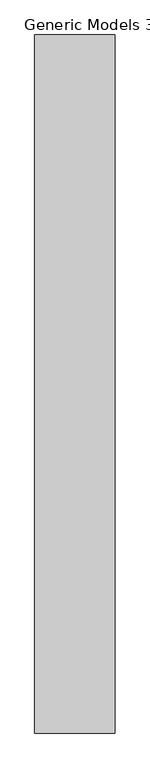
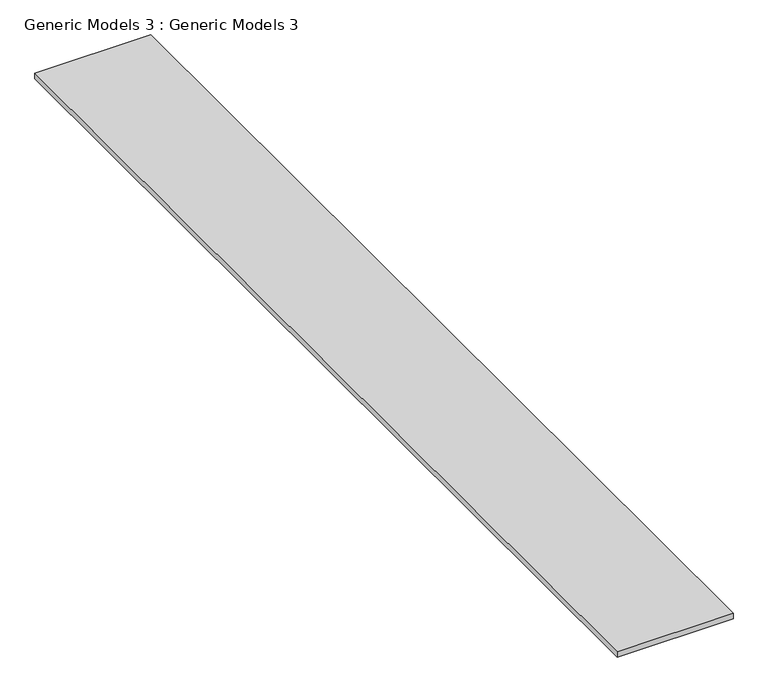
"""IFC4 building model written with IfcOpenShell, lengths in millimetres: proxy geometry, Generic Models 3 : Generic Models 3."""

from ifc_helpers import new_model, si_unit, frame, origin, place, context, project, spatial, polyline, outline, extrude, source, transform, mapped, element, save


def generic_models_3_generic_models_3_0a93b2c0(model_context):
    return source(origin(), model_context, "Body", "SweptSolid", [
        extrude(outline(polyline([(8005.385646, -11016.0591477), (8005.385646, 16286.4748919), (11143.9643979, 16286.4748919), (11143.9643979, -11016.0591477), (8005.385646, -11016.0591477)])), frame((0.0, 0.0, -152.4), z_axis=(0.0, 0.0, 1.0), x_axis=(1.0, 0.0, 0.0)), (0.0, 0.0, 1.0), 152.4),
    ])


if __name__ == "__main__":
    model = new_model("IFC4")
    model_context = context("Model", 3, world=origin())
    ifc_project = project(units=[si_unit("LENGTHUNIT", "METRE", prefix="MILLI")], contexts=[model_context])
    site = spatial("IfcSite", under=ifc_project)
    building = spatial("IfcBuilding", under=site)
    placement = place(None, origin())
    generic_models_3_generic_models_3_shape = generic_models_3_generic_models_3_0a93b2c0(model_context)
    element("IfcBuildingElementProxy", 1, Name="Generic Models 3 : Generic Models 3", ObjectType="Generic Models 3 : Generic Models 3", at=placement, inside=building, context=model_context, shape_type="MappedRepresentation", body=[
        mapped(generic_models_3_generic_models_3_shape, transform((0.0, 0.0, 0.0), x_axis=(1.0, 0.0, 0.0), y_axis=(0.0, 1.0, 0.0), z_axis=(0.0, 0.0, 1.0))),
    ])
    save(model, "model.ifc")
